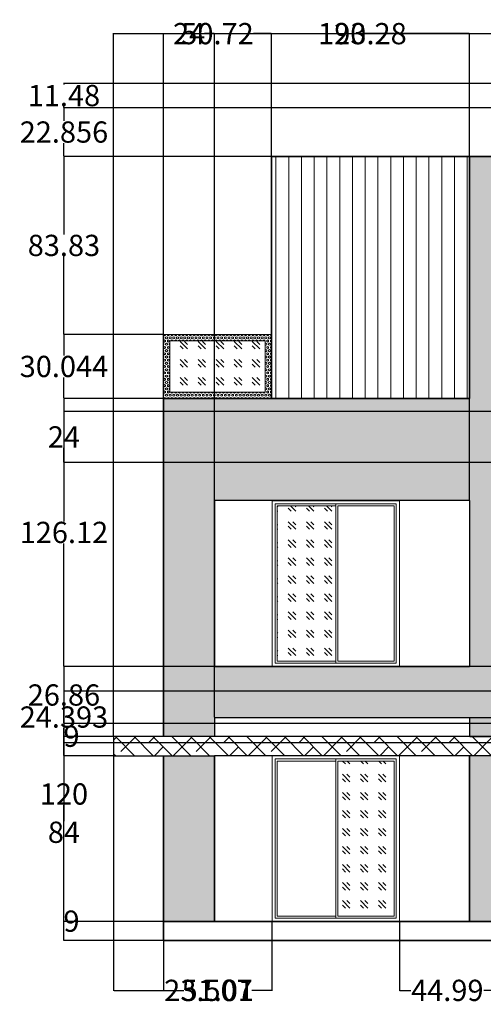
# Model space of a CAD drawing. Units: inches. Extents: x -37 to 519, y -28 to 435.
# Tile 1 of 3: x -37 to 182, y -28 to 435. Entities that reach past the tile are written whole.
import ezdxf

# ---------------------------------------------------------------- set-up
doc = ezdxf.new("R2010")
doc.units = ezdxf.units.IN
doc.header["$MEASUREMENT"] = 0
for name, color, linetype, lineweight in [('A-ANNO-DIMS', 2, 'Continuous', 18), ('A-GLAZ', 4, 'Continuous', 18), ('A-GLAZ-PATT', 9, 'Continuous', 13), ('A-WALL', 7, 'Continuous', 35), ('A-WALL-PATT', 8, 'Continuous', 13), ('A-WALL-TRIM', 7, 'Continuous', 25), ('A-WALL-TRIM-PATT', 8, 'Continuous', 13)]:
    doc.layers.add(name, color=color, linetype=linetype, lineweight=lineweight)
doc.styles.get("Standard").update_dxf_attribs({"font": 'arial.ttf'})
doc.dimstyles.get("Standard").update_dxf_attribs({"dimtxt": 10, "dimasz": 0.18, "dimexe": 0.18, "dimexo": 0.0625, "dimgap": 0.09, "dimtad": 0, "dimtih": 1, "dimtoh": 1, "dimdec": 0, "dimzin": 0, "dimdsep": 46, "dimlunit": 3, "dimtxsty": 'Standard', "dimcen": 0.09, "dimadec": 0, "dimazin": 0, "dimtfac": 1, "dimtdec": 0, "dimtofl": 0, "dimtmove": 0, "dimatfit": 3, "dimfxl": 1, "dimtolj": 1, "dimtzin": 0, "dimarcsym": 0})

# ---------------------------------------------------------------- blocks, each defined once
blk = doc.blocks.new('WIN-ALUM-60X78-ELEV')
for p, q in [((1.5, 1.5), (1.5, 76.5)), ((1.5, 76.5), (30, 76.5)), ((30, 1.5), (30, 76.5)), ((30, 76.5), (58.5, 76.5)), ((58.5, 76.5), (58.5, 1.5)), ((30, 1.5), (1.5, 1.5)), ((58.5, 1.5), (30, 1.5))]:
    blk.add_line(p, q)
blk.add_lwpolyline([(0, 0), (0, 78), (60, 78), (60, 0)], close=True)
for points in [[(29, 75.5), (29, 2.5), (2.5, 2.5), (2.5, 75.5), (29, 75.5)], [(30, 75.5), (57.5, 75.5), (57.5, 2.5), (30, 2.5)]]:
    blk.add_lwpolyline(points)
blk = doc.blocks.new('*D7')
at = {"layer": 'A-ANNO-DIMS', "color": 0, "lineweight": -2, "transparency": 16777216}
for p, q in [((7.62, 97.72), (7.62, 428.56)), ((7.8, 428.38), (224.17, 428.38)), ((474.95, 428.38), (258.57, 428.38)), ((475.13, 97.72), (475.13, 428.56))]:
    blk.add_line(p, q, dxfattribs=at)
at = {"layer": 'A-ANNO-DIMS', "color": 0, "transparency": 16777216}
for points in [[(7.8, 428.41), (7.8, 428.35), (7.62, 428.38)], [(474.95, 428.41), (474.95, 428.35), (475.13, 428.38)]]:
    blk.add_solid(points, dxfattribs=at)
at = {"layer": 'Defpoints', "color": 0, "transparency": 16777216}
for p in [(475.13, 428.38), (7.62, 97.65), (475.13, 97.65)]:
    blk.add_point(p, dxfattribs=at)
at = {"layer": 'A-ANNO-DIMS', "color": 0, "transparency": 16777216, "insert": (241.37, 428.38), "char_height": 10, "attachment_point": 5}
blk.add_mtext('\\A1;467.5', dxfattribs=at)
blk = doc.blocks.new('*D9')
at = {"layer": 'A-ANNO-DIMS', "color": 0, "lineweight": -2, "transparency": 16777216}
for p, q in [((7.62, 88.59), (7.62, -21.92)), ((31.13, 1.59), (31.13, -21.92)), ((7.8, -21.74), (30.95, -21.74)), ((31.13, -21.74), (31.31, -21.74))]:
    blk.add_line(p, q, dxfattribs=at)
at = {"layer": 'A-ANNO-DIMS', "color": 0, "transparency": 16777216}
for points in [[(7.8, -21.71), (7.8, -21.77), (7.62, -21.74)], [(30.95, -21.71), (30.95, -21.77), (31.13, -21.74)]]:
    blk.add_solid(points, dxfattribs=at)
at = {"layer": 'Defpoints', "color": 0, "transparency": 16777216}
for p in [(7.62, 88.65), (31.13, 1.65), (31.13, -21.74)]:
    blk.add_point(p, dxfattribs=at)
at = {"layer": 'A-ANNO-DIMS', "color": 0, "transparency": 16777216, "insert": (52.24, -21.74), "char_height": 10, "attachment_point": 5}
blk.add_mtext('\\A1;23.507', dxfattribs=at)
blk = doc.blocks.new('*D10')
at = {"layer": 'A-ANNO-DIMS', "color": 0, "lineweight": -2, "transparency": 16777216}
for p, q in [((31.13, 10.59), (31.13, -21.92)), ((82.13, 10.59), (82.13, -21.92)), ((31.31, -21.74), (40.63, -21.74)), ((81.95, -21.74), (72.63, -21.74))]:
    blk.add_line(p, q, dxfattribs=at)
at = {"layer": 'A-ANNO-DIMS', "color": 0, "transparency": 16777216}
for points in [[(31.31, -21.71), (31.31, -21.77), (31.13, -21.74)], [(81.95, -21.71), (81.95, -21.77), (82.13, -21.74)]]:
    blk.add_solid(points, dxfattribs=at)
at = {"layer": 'Defpoints', "color": 0, "transparency": 16777216}
for p in [(31.13, 10.65), (82.13, 10.65), (82.13, -21.74)]:
    blk.add_point(p, dxfattribs=at)
at = {"layer": 'A-ANNO-DIMS', "color": 0, "transparency": 16777216, "insert": (56.63, -21.74), "char_height": 10, "attachment_point": 5}
blk.add_mtext('\\A1;51.01', dxfattribs=at)
blk = doc.blocks.new('*D11')
at = {"layer": 'A-ANNO-DIMS', "color": 0, "lineweight": -2, "transparency": 16777216}
for p, q in [((142.13, 10.59), (142.13, -21.92)), ((187.13, 10.59), (187.13, -21.92)), ((142.31, -21.74), (147.46, -21.74)), ((186.95, -21.74), (181.8, -21.74))]:
    blk.add_line(p, q, dxfattribs=at)
at = {"layer": 'A-ANNO-DIMS', "color": 0, "transparency": 16777216}
for points in [[(142.31, -21.71), (142.31, -21.77), (142.13, -21.74)], [(186.95, -21.71), (186.95, -21.77), (187.13, -21.74)]]:
    blk.add_solid(points, dxfattribs=at)
at = {"layer": 'Defpoints', "color": 0, "transparency": 16777216}
for p in [(142.13, 10.65), (187.13, 10.65), (187.13, -21.74)]:
    blk.add_point(p, dxfattribs=at)
at = {"layer": 'A-ANNO-DIMS', "color": 0, "transparency": 16777216, "insert": (164.63, -21.74), "char_height": 10, "attachment_point": 5}
blk.add_mtext('\\A1;44.99', dxfattribs=at)
blk = doc.blocks.new('*D16')
at = {"layer": 'A-ANNO-DIMS', "color": 0, "lineweight": -2, "transparency": 16777216}
for p, q in [((206.27, 94.65), (-15.95, 94.65)), ((-15.77, 94.47), (-15.77, 57.85)), ((-15.77, 10.83), (-15.77, 47.46)), ((206.27, 10.65), (-15.95, 10.65))]:
    blk.add_line(p, q, dxfattribs=at)
at = {"layer": 'A-ANNO-DIMS', "color": 0, "transparency": 16777216}
for points in [[(-15.8, 94.47), (-15.74, 94.47), (-15.77, 94.65)], [(-15.8, 10.83), (-15.74, 10.83), (-15.77, 10.65)]]:
    blk.add_solid(points, dxfattribs=at)
at = {"layer": 'Defpoints', "color": 0, "transparency": 16777216}
for p in [(-15.77, 94.65), (206.33, 94.65), (206.33, 10.65)]:
    blk.add_point(p, dxfattribs=at)
at = {"layer": 'A-ANNO-DIMS', "color": 0, "transparency": 16777216, "insert": (-15.77, 52.65), "char_height": 10, "attachment_point": 5}
blk.add_mtext('\\A1;84', dxfattribs=at)
blk = doc.blocks.new('*D18')
at = {"layer": 'A-ANNO-DIMS', "color": 0, "lineweight": -2, "transparency": 16777216}
for p, q in [((31.06, 10.65), (-15.95, 10.65)), ((-15.77, 10.65), (-15.77, 10.83)), ((-15.77, 10.83), (-15.59, 10.83)), ((-15.77, 1.83), (-15.77, 10.47)), ((31.06, 1.65), (-15.95, 1.65))]:
    blk.add_line(p, q, dxfattribs=at)
at = {"layer": 'A-ANNO-DIMS', "color": 0, "transparency": 16777216}
for points in [[(-15.8, 10.47), (-15.74, 10.47), (-15.77, 10.65)], [(-15.8, 1.83), (-15.74, 1.83), (-15.77, 1.65)]]:
    blk.add_solid(points, dxfattribs=at)
at = {"layer": 'Defpoints', "color": 0, "transparency": 16777216}
for p in [(-15.77, 10.65), (31.13, 10.65), (31.13, 1.65)]:
    blk.add_point(p, dxfattribs=at)
at = {"layer": 'A-ANNO-DIMS', "color": 0, "transparency": 16777216, "insert": (-12.21, 10.83), "char_height": 10, "attachment_point": 5}
blk.add_mtext('\\A1;9', dxfattribs=at)
blk = doc.blocks.new('*D19')
at = {"layer": 'A-ANNO-DIMS', "color": 0, "lineweight": -2, "transparency": 16777216}
for p, q in [((82.07, 130.65), (-15.95, 130.65)), ((-15.77, 130.47), (-15.77, 75.85)), ((-15.77, 10.83), (-15.77, 65.46)), ((31.06, 10.65), (-15.95, 10.65))]:
    blk.add_line(p, q, dxfattribs=at)
at = {"layer": 'A-ANNO-DIMS', "color": 0, "transparency": 16777216}
for points in [[(-15.8, 130.47), (-15.74, 130.47), (-15.77, 130.65)], [(-15.8, 10.83), (-15.74, 10.83), (-15.77, 10.65)]]:
    blk.add_solid(points, dxfattribs=at)
at = {"layer": 'Defpoints', "color": 0, "transparency": 16777216}
for p in [(-15.77, 130.65), (82.13, 130.65), (31.13, 10.65)]:
    blk.add_point(p, dxfattribs=at)
at = {"layer": 'A-ANNO-DIMS', "color": 0, "transparency": 16777216, "insert": (-15.77, 70.65), "char_height": 10, "attachment_point": 5}
blk.add_mtext('\\A1;120', dxfattribs=at)
blk = doc.blocks.new('*D20')
at = {"layer": 'A-ANNO-DIMS', "color": 0, "lineweight": -2, "transparency": 16777216}
for p, q in [((31.06, 256.78), (-15.95, 256.78)), ((-15.77, 256.6), (-15.77, 198.91)), ((-15.77, 130.83), (-15.77, 188.52)), ((82.07, 130.65), (-15.95, 130.65))]:
    blk.add_line(p, q, dxfattribs=at)
at = {"layer": 'A-ANNO-DIMS', "color": 0, "transparency": 16777216}
for points in [[(-15.8, 256.6), (-15.74, 256.6), (-15.77, 256.78)], [(-15.8, 130.83), (-15.74, 130.83), (-15.77, 130.65)]]:
    blk.add_solid(points, dxfattribs=at)
at = {"layer": 'Defpoints', "color": 0, "transparency": 16777216}
for p in [(-15.77, 256.78), (31.13, 256.78), (82.13, 130.65)]:
    blk.add_point(p, dxfattribs=at)
at = {"layer": 'A-ANNO-DIMS', "color": 0, "transparency": 16777216, "insert": (-15.77, 193.71), "char_height": 10, "attachment_point": 5}
blk.add_mtext('\\A1;126.12', dxfattribs=at)
blk = doc.blocks.new('*D21')
at = {"layer": 'A-ANNO-DIMS', "color": 0, "lineweight": -2, "transparency": 16777216}
for p, q in [((31.06, 286.82), (-15.95, 286.82)), ((-15.77, 286.64), (-15.77, 277)), ((-15.77, 256.96), (-15.77, 266.6)), ((31.06, 256.78), (-15.95, 256.78))]:
    blk.add_line(p, q, dxfattribs=at)
at = {"layer": 'A-ANNO-DIMS', "color": 0, "transparency": 16777216}
for points in [[(-15.8, 286.64), (-15.74, 286.64), (-15.77, 286.82)], [(-15.8, 256.96), (-15.74, 256.96), (-15.77, 256.78)]]:
    blk.add_solid(points, dxfattribs=at)
at = {"layer": 'Defpoints', "color": 0, "transparency": 16777216}
for p in [(-15.77, 286.82), (31.13, 286.82), (31.13, 256.78)]:
    blk.add_point(p, dxfattribs=at)
at = {"layer": 'A-ANNO-DIMS', "color": 0, "transparency": 16777216, "insert": (-15.77, 271.8), "char_height": 10, "attachment_point": 5}
blk.add_mtext('\\A1;30.044', dxfattribs=at)
blk = doc.blocks.new('*D22')
at = {"layer": 'A-ANNO-DIMS', "color": 0, "lineweight": -2, "transparency": 16777216}
for p, q in [((81.79, 370.65), (-15.95, 370.65)), ((-15.77, 370.47), (-15.77, 333.94)), ((-15.77, 287), (-15.77, 323.54)), ((31.06, 286.82), (-15.95, 286.82))]:
    blk.add_line(p, q, dxfattribs=at)
at = {"layer": 'A-ANNO-DIMS', "color": 0, "transparency": 16777216}
for points in [[(-15.8, 370.47), (-15.74, 370.47), (-15.77, 370.65)], [(-15.8, 287), (-15.74, 287), (-15.77, 286.82)]]:
    blk.add_solid(points, dxfattribs=at)
at = {"layer": 'Defpoints', "color": 0, "transparency": 16777216}
for p in [(-15.77, 370.65), (81.85, 370.65), (31.13, 286.82)]:
    blk.add_point(p, dxfattribs=at)
at = {"layer": 'A-ANNO-DIMS', "color": 0, "transparency": 16777216, "insert": (-15.77, 328.74), "char_height": 10, "attachment_point": 5}
blk.add_mtext('\\A1;83.83', dxfattribs=at)
blk = doc.blocks.new('*D23')
at = {"layer": 'A-ANNO-DIMS', "color": 0, "lineweight": -2, "transparency": 16777216}
for p, q in [((31.13, 286.88), (31.13, 428.56)), ((31.31, 428.38), (39.58, 428.38)), ((81.67, 428.38), (73.4, 428.38)), ((81.85, 370.72), (81.85, 428.56))]:
    blk.add_line(p, q, dxfattribs=at)
at = {"layer": 'A-ANNO-DIMS', "color": 0, "transparency": 16777216}
for points in [[(31.31, 428.41), (31.31, 428.35), (31.13, 428.38)], [(81.67, 428.41), (81.67, 428.35), (81.85, 428.38)]]:
    blk.add_solid(points, dxfattribs=at)
at = {"layer": 'Defpoints', "color": 0, "transparency": 16777216}
for p in [(81.85, 428.38), (81.85, 370.65), (31.13, 286.82)]:
    blk.add_point(p, dxfattribs=at)
at = {"layer": 'A-ANNO-DIMS', "color": 0, "transparency": 16777216, "insert": (56.49, 428.38), "char_height": 10, "attachment_point": 5}
blk.add_mtext('\\A1;50.72', dxfattribs=at)
blk = doc.blocks.new('*D24')
at = {"layer": 'A-ANNO-DIMS', "color": 0, "lineweight": -2, "transparency": 16777216}
for p, q in [((81.85, 370.72), (81.85, 428.56)), ((82.03, 428.38), (111.52, 428.38)), ((174.95, 428.38), (145.46, 428.38)), ((175.13, 370.72), (175.13, 428.56))]:
    blk.add_line(p, q, dxfattribs=at)
at = {"layer": 'A-ANNO-DIMS', "color": 0, "transparency": 16777216}
for points in [[(82.03, 428.41), (82.03, 428.35), (81.85, 428.38)], [(174.95, 428.41), (174.95, 428.35), (175.13, 428.38)]]:
    blk.add_solid(points, dxfattribs=at)
at = {"layer": 'Defpoints', "color": 0, "transparency": 16777216}
for p in [(175.13, 428.38), (81.85, 370.65), (175.13, 370.65)]:
    blk.add_point(p, dxfattribs=at)
at = {"layer": 'A-ANNO-DIMS', "color": 0, "transparency": 16777216, "insert": (128.49, 428.38), "char_height": 10, "attachment_point": 5}
blk.add_mtext('\\A1;93.28', dxfattribs=at)
blk = doc.blocks.new('*D27')
at = {"layer": 'A-ANNO-DIMS', "color": 0, "lineweight": -2, "transparency": 16777216}
for p, q in [((295.06, 119.05), (-15.95, 119.05)), ((-15.77, 118.87), (-15.77, 112.05)), ((-15.77, 94.83), (-15.77, 101.65)), ((266, 94.65), (-15.95, 94.65))]:
    blk.add_line(p, q, dxfattribs=at)
at = {"layer": 'A-ANNO-DIMS', "color": 0, "transparency": 16777216}
for points in [[(-15.8, 118.87), (-15.74, 118.87), (-15.77, 119.05)], [(-15.8, 94.83), (-15.74, 94.83), (-15.77, 94.65)]]:
    blk.add_solid(points, dxfattribs=at)
at = {"layer": 'Defpoints', "color": 0, "transparency": 16777216}
for p in [(-15.77, 119.05), (295.13, 119.05), (266.06, 94.65)]:
    blk.add_point(p, dxfattribs=at)
at = {"layer": 'A-ANNO-DIMS', "color": 0, "transparency": 16777216, "insert": (-15.77, 106.85), "char_height": 10, "attachment_point": 5}
blk.add_mtext('\\A1;24.393', dxfattribs=at)
blk = doc.blocks.new('*D28')
at = {"layer": 'A-ANNO-DIMS', "color": 0, "lineweight": -2, "transparency": 16777216}
for p, q in [((7.56, 97.65), (-15.95, 97.65)), ((-15.77, 97.65), (-15.77, 97.83)), ((-15.77, 97.83), (-15.59, 97.83)), ((-15.77, 88.83), (-15.77, 97.47)), ((7.56, 88.65), (-15.95, 88.65))]:
    blk.add_line(p, q, dxfattribs=at)
at = {"layer": 'A-ANNO-DIMS', "color": 0, "transparency": 16777216}
for points in [[(-15.8, 97.47), (-15.74, 97.47), (-15.77, 97.65)], [(-15.8, 88.83), (-15.74, 88.83), (-15.77, 88.65)]]:
    blk.add_solid(points, dxfattribs=at)
at = {"layer": 'Defpoints', "color": 0, "transparency": 16777216}
for p in [(-15.77, 97.65), (7.62, 97.65), (7.62, 88.65)]:
    blk.add_point(p, dxfattribs=at)
at = {"layer": 'A-ANNO-DIMS', "color": 0, "transparency": 16777216, "insert": (-12.21, 97.83), "char_height": 10, "attachment_point": 5}
blk.add_mtext('\\A1;9', dxfattribs=at)
blk = doc.blocks.new('*D29')
at = {"layer": 'A-ANNO-DIMS', "color": 0, "lineweight": -2, "transparency": 16777216}
for p, q in [((55.13, 208.84), (55.13, 428.56)), ((55.31, 428.38), (104.48, 428.38)), ((174.95, 428.38), (125.78, 428.38)), ((175.13, 208.84), (175.13, 428.56))]:
    blk.add_line(p, q, dxfattribs=at)
at = {"layer": 'A-ANNO-DIMS', "color": 0, "transparency": 16777216}
for points in [[(55.31, 428.41), (55.31, 428.35), (55.13, 428.38)], [(174.95, 428.41), (174.95, 428.35), (175.13, 428.38)]]:
    blk.add_solid(points, dxfattribs=at)
at = {"layer": 'Defpoints', "color": 0, "transparency": 16777216}
for p in [(175.13, 428.38), (55.13, 208.78), (175.13, 208.78)]:
    blk.add_point(p, dxfattribs=at)
at = {"layer": 'A-ANNO-DIMS', "color": 0, "transparency": 16777216, "insert": (115.13, 428.38), "char_height": 10, "attachment_point": 5}
blk.add_mtext('\\A1;120', dxfattribs=at)
blk = doc.blocks.new('*D30')
at = {"layer": 'A-ANNO-DIMS', "color": 0, "lineweight": -2, "transparency": 16777216}
for p, q in [((31.13, 97.72), (31.13, 428.56)), ((31.31, 428.38), (35.81, 428.38)), ((54.95, 428.38), (50.44, 428.38)), ((55.13, 106.72), (55.13, 428.56))]:
    blk.add_line(p, q, dxfattribs=at)
at = {"layer": 'A-ANNO-DIMS', "color": 0, "transparency": 16777216}
for points in [[(31.31, 428.41), (31.31, 428.35), (31.13, 428.38)], [(54.95, 428.41), (54.95, 428.35), (55.13, 428.38)]]:
    blk.add_solid(points, dxfattribs=at)
at = {"layer": 'Defpoints', "color": 0, "transparency": 16777216}
for p in [(55.13, 428.38), (55.13, 106.65), (31.13, 97.65)]:
    blk.add_point(p, dxfattribs=at)
at = {"layer": 'A-ANNO-DIMS', "color": 0, "transparency": 16777216, "insert": (43.13, 428.38), "char_height": 10, "attachment_point": 5}
blk.add_mtext('\\A1;24', dxfattribs=at)
blk = doc.blocks.new('*D31')
at = {"layer": 'A-ANNO-DIMS', "color": 0, "lineweight": -2, "transparency": 16777216}
for p, q in [((175.19, 106.65), (498.7, 106.65)), ((498.52, 106.65), (498.52, 106.83)), ((498.52, 106.83), (498.7, 106.83)), ((498.52, 97.83), (498.52, 106.47)), ((175.19, 97.65), (498.7, 97.65))]:
    blk.add_line(p, q, dxfattribs=at)
at = {"layer": 'A-ANNO-DIMS', "color": 0, "transparency": 16777216}
for points in [[(498.49, 106.47), (498.55, 106.47), (498.52, 106.65)], [(498.49, 97.83), (498.55, 97.83), (498.52, 97.65)]]:
    blk.add_solid(points, dxfattribs=at)
at = {"layer": 'Defpoints', "color": 0, "transparency": 16777216}
for p in [(175.13, 106.65), (498.52, 106.65), (175.13, 97.65)]:
    blk.add_point(p, dxfattribs=at)
at = {"layer": 'A-ANNO-DIMS', "color": 0, "transparency": 16777216, "insert": (502.08, 106.83), "char_height": 10, "attachment_point": 5}
blk.add_mtext('\\A1;9', dxfattribs=at)
blk = doc.blocks.new('*D33')
at = {"layer": 'A-ANNO-DIMS', "color": 0, "lineweight": -2, "transparency": 16777216}
for p, q in [((319.06, 250.65), (-15.95, 250.65)), ((-15.77, 250.47), (-15.77, 243.76)), ((-15.77, 226.83), (-15.77, 233.54)), ((295.06, 226.65), (-15.95, 226.65))]:
    blk.add_line(p, q, dxfattribs=at)
at = {"layer": 'A-ANNO-DIMS', "color": 0, "transparency": 16777216}
for points in [[(-15.8, 250.47), (-15.74, 250.47), (-15.77, 250.65)], [(-15.8, 226.83), (-15.74, 226.83), (-15.77, 226.65)]]:
    blk.add_solid(points, dxfattribs=at)
at = {"layer": 'Defpoints', "color": 0, "transparency": 16777216}
for p in [(319.13, 250.65), (-15.77, 226.65), (295.13, 226.65)]:
    blk.add_point(p, dxfattribs=at)
at = {"layer": 'A-ANNO-DIMS', "color": 0, "transparency": 16777216, "insert": (-15.77, 238.65), "char_height": 10, "attachment_point": 5}
blk.add_mtext('\\A1;24', dxfattribs=at)
blk = doc.blocks.new('*D42')
at = {"layer": 'A-ANNO-DIMS', "color": 0, "lineweight": -2, "transparency": 16777216}
for p, q in [((312.44, 393.51), (-15.95, 393.51)), ((-15.77, 393.33), (-15.77, 387.28)), ((-15.77, 370.83), (-15.77, 376.89)), ((312.44, 370.65), (-15.95, 370.65))]:
    blk.add_line(p, q, dxfattribs=at)
at = {"layer": 'A-ANNO-DIMS', "color": 0, "transparency": 16777216}
for points in [[(-15.8, 393.33), (-15.74, 393.33), (-15.77, 393.51)], [(-15.8, 370.83), (-15.74, 370.83), (-15.77, 370.65)]]:
    blk.add_solid(points, dxfattribs=at)
at = {"layer": 'Defpoints', "color": 0, "transparency": 16777216}
for p in [(-15.77, 393.51), (312.5, 393.51), (312.5, 370.65)]:
    blk.add_point(p, dxfattribs=at)
at = {"layer": 'A-ANNO-DIMS', "color": 0, "transparency": 16777216, "insert": (-15.77, 382.08), "char_height": 10, "attachment_point": 5}
blk.add_mtext('\\A1;22.856', dxfattribs=at)
blk = doc.blocks.new('*D43')
at = {"layer": 'A-ANNO-DIMS', "color": 0, "lineweight": -2, "transparency": 16777216}
for p, q in [((295.06, 404.99), (-15.95, 404.99)), ((-15.77, 404.81), (-15.77, 404.44)), ((-15.77, 393.69), (-15.77, 394.05)), ((295.06, 393.51), (-15.95, 393.51))]:
    blk.add_line(p, q, dxfattribs=at)
at = {"layer": 'A-ANNO-DIMS', "color": 0, "transparency": 16777216}
for points in [[(-15.8, 404.81), (-15.74, 404.81), (-15.77, 404.99)], [(-15.8, 393.69), (-15.74, 393.69), (-15.77, 393.51)]]:
    blk.add_solid(points, dxfattribs=at)
at = {"layer": 'Defpoints', "color": 0, "transparency": 16777216}
for p in [(-15.77, 404.99), (295.13, 404.99), (295.13, 393.51)]:
    blk.add_point(p, dxfattribs=at)
at = {"layer": 'A-ANNO-DIMS', "color": 0, "transparency": 16777216, "insert": (-15.77, 399.25), "char_height": 10, "attachment_point": 5}
blk.add_mtext('\\A1;11.48', dxfattribs=at)
blk = doc.blocks.new('*D46')
at = {"layer": 'A-ANNO-DIMS', "color": 0, "lineweight": -2, "transparency": 16777216}
for p, q in [((307.06, 130.65), (-15.95, 130.65)), ((-15.77, 130.47), (-15.77, 122.42)), ((-15.77, 103.97), (-15.77, 112.03)), ((307.06, 103.79), (-15.95, 103.79))]:
    blk.add_line(p, q, dxfattribs=at)
at = {"layer": 'A-ANNO-DIMS', "color": 0, "transparency": 16777216}
for points in [[(-15.8, 130.47), (-15.74, 130.47), (-15.77, 130.65)], [(-15.8, 103.97), (-15.74, 103.97), (-15.77, 103.79)]]:
    blk.add_solid(points, dxfattribs=at)
at = {"layer": 'Defpoints', "color": 0, "transparency": 16777216}
for p in [(307.13, 130.65), (-15.77, 103.79), (307.13, 103.79)]:
    blk.add_point(p, dxfattribs=at)
at = {"layer": 'A-ANNO-DIMS', "color": 0, "transparency": 16777216, "insert": (-15.77, 117.22), "char_height": 10, "attachment_point": 5}
blk.add_mtext('\\A1;26.86', dxfattribs=at)

msp = doc.modelspace()

# ---------------------------------------------------------------- hatches: boundary and pattern name
at = {"layer": 'A-GLAZ-PATT'}
h = msp.add_hatch(dxfattribs=at)
h.set_pattern_fill('GOST_GLASS', color=256, angle=90)
h.set_pattern_definition([(135, (0, 0), (5e-16, 8.48528), [5, -7]), (135, (1e-16, 2.1213), (5e-16, 8.48528), [2, -10]), (135, (-2.1213, 1e-16), (5e-16, 8.48528), [2, -10])])
h.paths.add_polyline_path([(112.1341, 206.153), (84.6341, 206.153), (84.6341, 133.153), (112.1341, 133.153)])
h.paths.add_polyline_path([(139.6341, 86.153), (113.1341, 86.153), (113.1341, 13.153), (139.6341, 13.153)])
h.paths.add_polyline_path([(369.1204, 86.153), (342.6204, 86.153), (342.6204, 13.153), (369.1204, 13.153)])
h.paths.add_polyline_path([(391.6341, 206.153), (365.1341, 206.153), (365.1341, 133.153), (391.6341, 133.153)])
h.paths.add_polyline_path([(78.851, 283.8209), (34.1272, 283.8209), (34.1272, 259.7765), (78.851, 259.7765)])
at = {"layer": 'A-WALL-PATT'}
h = msp.add_hatch(color=256, dxfattribs=at)
h.dxf.hatch_style = 1
h.paths.add_polyline_path([(451.1272, 370.653), (295.1272, 370.653), (295.1272, 226.653), (451.1272, 226.653)])
h.paths.add_polyline_path([(319.1272, 346.653), (427.1272, 346.653), (427.1272, 250.653), (319.1272, 250.653)], flags=16)
h.paths.add_polyline_path([(334.1341, 346.653), (394.1341, 346.653), (394.1341, 250.653), (334.1341, 250.653)], flags=0)
h.paths.add_polyline_path([(335.6341, 345.153), (364.1341, 345.153), (392.6341, 345.153), (392.6341, 252.153), (364.1341, 252.153), (335.6341, 252.153)], flags=0)
h.paths.add_polyline_path([(336.6341, 344.153), (364.1341, 344.153), (364.1341, 253.153), (336.6341, 253.153)], flags=0)
h.paths.add_polyline_path([(365.1341, 344.153), (391.6341, 344.153), (391.6341, 253.153), (365.1341, 253.153)], flags=0)
h.paths.add_polyline_path([(187.1272, 370.653), (175.1272, 370.653), (175.1272, 256.7765), (31.1272, 256.7765), (31.1272, 97.653), (55.1272, 97.653), (55.1272, 106.653), (175.1272, 106.653), (175.1272, 97.653), (187.1272, 97.653)])
h.paths.add_polyline_path([(175.1272, 208.7765), (175.1272, 130.653), (55.1272, 130.653), (55.1272, 208.7765)], flags=16)
h.paths.add_polyline_path([(142.1341, 208.653), (142.1341, 130.653), (82.1341, 130.653), (82.1341, 208.653)], flags=0)
h.paths.add_polyline_path([(112.1341, 207.153), (140.6341, 207.153), (140.6341, 132.153), (112.1341, 132.153), (83.6341, 132.153), (83.6341, 207.153)], flags=0)
h.paths.add_polyline_path([(112.1341, 133.153), (84.6341, 133.153), (84.6341, 206.153), (112.1341, 206.153)], flags=0)
h.paths.add_polyline_path([(139.6341, 206.153), (139.6341, 133.153), (113.1341, 133.153), (113.1341, 206.153)], flags=0)
h.paths.add_polyline_path([(187.1272, 88.653), (175.1272, 88.653), (175.1272, 10.653), (187.1272, 10.653)])
h.paths.add_polyline_path([(307.1272, 88.653), (295.1272, 88.653), (295.1272, 10.653), (307.1272, 10.653)])
h.paths.add_polyline_path([(451.1272, 88.653), (427.1272, 88.653), (427.1272, 10.653), (451.1272, 10.653)])
h = msp.add_hatch(dxfattribs=at)
h.set_pattern_fill('_USER', color=256, scale=6, angle=90, pattern_type=0)
h.set_pattern_definition([(90, (0, 0), (-6, 4e-16), [])])
h.paths.add_polyline_path([(175.1272, 370.653), (81.851, 370.653), (81.851, 256.7765), (175.1272, 256.7765)])
h = msp.add_hatch(color=256, dxfattribs=at)
h.dxf.hatch_style = 1
h.paths.add_polyline_path([(307.1272, 226.653), (295.1272, 226.653), (295.1272, 97.653), (307.1272, 97.653), (307.1272, 130.653)])
h.paths.add_polyline_path([(55.1272, 88.653), (31.1272, 88.653), (31.1272, 10.653), (55.1272, 10.653)])
at = {"layer": 'A-WALL-TRIM-PATT'}
h = msp.add_hatch(dxfattribs=at)
h.set_pattern_fill('HEX', color=256, scale=4, angle=90)
h.paths.add_polyline_path([(81.851, 286.8209), (31.1272, 286.8209), (31.1272, 256.7765), (81.851, 256.7765)])
h.paths.add_polyline_path([(78.851, 283.8209), (78.851, 259.7765), (34.1272, 259.7765), (34.1272, 283.8209)], flags=16)
h = msp.add_hatch(dxfattribs=at)
h.set_pattern_fill('ANSI38', color=256, scale=50, angle=90)
h.paths.add_polyline_path([(187.1272, 97.653), (55.1272, 97.653), (7.6202, 97.653), (7.6202, 88.653), (55.1272, 88.653), (187.1272, 88.653)])
h.paths.add_polyline_path([(475.1272, 97.653), (427.1272, 97.653), (295.1272, 97.653), (295.1272, 88.653), (427.1272, 88.653), (475.1272, 88.653)])

# ---------------------------------------------------------------- linework, layer by layer
at = {"layer": 'A-GLAZ'}
for p, q in [((112.1341, 207.153), (83.6341, 207.153)), ((83.6341, 207.153), (83.6341, 132.153)), ((112.1341, 132.153), (112.1341, 207.153)), ((140.6341, 207.153), (112.1341, 207.153)), ((140.6341, 132.153), (140.6341, 207.153)), ((83.6341, 132.153), (112.1341, 132.153)), ((112.1341, 132.153), (140.6341, 132.153)), ((112.1341, 87.153), (83.6341, 87.153)), ((83.6341, 87.153), (83.6341, 12.153)), ((112.1341, 12.153), (112.1341, 87.153)), ((140.6341, 87.153), (112.1341, 87.153)), ((140.6341, 12.153), (140.6341, 87.153)), ((83.6341, 12.153), (112.1341, 12.153)), ((112.1341, 12.153), (140.6341, 12.153))]:
    msp.add_line(p, q, dxfattribs=at)
for points in [[(81.851, 286.8209), (31.1272, 286.8209), (31.1272, 256.7765), (81.851, 256.7765)], [(78.851, 283.8209), (34.1272, 283.8209), (34.1272, 259.7765), (78.851, 259.7765)], [(142.1341, 130.653), (142.1341, 208.653), (82.1341, 208.653), (82.1341, 130.653)], [(142.1341, 10.653), (142.1341, 88.653), (82.1341, 88.653), (82.1341, 10.653)]]:
    msp.add_lwpolyline(points, close=True, dxfattribs=at)
for points in [[(112.1341, 206.153), (84.6341, 206.153), (84.6341, 133.153), (112.1341, 133.153)], [(113.1341, 206.153), (113.1341, 133.153), (139.6341, 133.153), (139.6341, 206.153), (113.1341, 206.153)], [(112.1341, 86.153), (84.6341, 86.153), (84.6341, 13.153), (112.1341, 13.153)], [(113.1341, 86.153), (113.1341, 13.153), (139.6341, 13.153), (139.6341, 86.153), (113.1341, 86.153)]]:
    msp.add_lwpolyline(points, dxfattribs=at)
at = {"layer": 'A-WALL'}
for p, q in [((81.851, 370.653), (81.851, 256.7765)), ((187.1272, 370.653), (81.851, 370.653)), ((175.1272, 370.653), (175.1272, 256.7765)), ((31.1272, 256.7765), (31.1272, 97.653)), ((175.1272, 256.7765), (31.1272, 256.7765)), ((31.1272, 88.653), (31.1272, 1.653)), ((55.1272, 88.653), (55.1272, 10.653)), ((175.1272, 88.653), (175.1272, 10.653)), ((31.1272, 10.653), (451.1272, 10.653)), ((31.1272, 1.653), (451.1272, 1.653))]:
    msp.add_line(p, q, dxfattribs=at)
at = {"layer": 'A-WALL-TRIM'}
for p, q in [((55.1272, 208.7765), (55.1272, 130.653)), ((175.1272, 208.7765), (55.1272, 208.7765)), ((175.1272, 208.7765), (175.1272, 130.653)), ((55.1272, 130.653), (163.1272, 130.653)), ((55.1272, 130.653), (175.1272, 130.653)), ((55.1272, 106.653), (163.1272, 106.653)), ((55.1272, 106.653), (175.1272, 106.653)), ((55.1272, 106.653), (55.1272, 97.653)), ((175.1272, 106.653), (175.1272, 97.653)), ((187.1272, 97.653), (55.1272, 97.653)), ((187.1272, 88.653), (55.1272, 88.653))]:
    msp.add_line(p, q, dxfattribs=at)
msp.add_lwpolyline([(55.1272, 97.653), (7.6202, 97.653), (7.6202, 88.653), (55.1272, 88.653)], dxfattribs=at)

# ---------------------------------------------------------------- block references
at = {"layer": 'A-GLAZ', "extrusion": (0, 0, -1), "zscale": -1}
for p in [(-142.1341, 130.653), (-142.1341, 10.653)]:
    msp.add_blockref('WIN-ALUM-60X78-ELEV', p, dxfattribs=at)

# ---------------------------------------------------------------- dimensions: what is measured, and where the dimension line sits
at = {"layer": 'A-ANNO-DIMS'}
for base, p1, p2, override, picture, middle in [((475.1272, 428.3793), (7.6202, 97.653), (475.1272, 97.653), {"dimdec": 1, "dimlfac": 1, "dimrnd": 0, "dimzin": 0, "dimdsep": 46, "dimlunit": 2}, '*D7', (241.3737, 428.3793)), ((81.851, 428.3793), (31.1272, 286.8209), (81.851, 370.653), {"dimdec": 2, "dimlfac": 1, "dimrnd": 0, "dimzin": 0, "dimdsep": 46, "dimlunit": 2}, '*D23', (56.4891, 428.3793)), ((55.1272, 428.3793), (31.1272, 97.653), (55.1272, 106.653), {"dimdec": 0, "dimlfac": 1, "dimrnd": 0, "dimzin": 0, "dimdsep": 46, "dimlunit": 2}, '*D30', (43.1272, 428.3793)), ((175.1272, 428.3793), (55.1272, 208.7765), (175.1272, 208.7765), {"dimdec": 0, "dimlfac": 1, "dimrnd": 0, "dimzin": 0, "dimdsep": 46, "dimlunit": 2}, '*D29', (115.1272, 428.3793)), ((175.1272, 428.3793), (81.851, 370.653), (175.1272, 370.653), {"dimdec": 2, "dimlfac": 1, "dimrnd": 0, "dimzin": 0, "dimdsep": 46, "dimlunit": 2}, '*D24', (128.4891, 428.3793)), ((31.1272, -21.737), (7.6202, 88.653), (31.1272, 1.653), {"dimdec": 3, "dimlfac": 1, "dimrnd": 0, "dimzin": 0, "dimdsep": 46, "dimlunit": 2}, '*D9', (52.2397, -21.737)), ((82.1341, -21.737), (31.1272, 10.653), (82.1341, 10.653), {"dimdec": 2, "dimlfac": 1, "dimrnd": 0, "dimzin": 0, "dimdsep": 46, "dimlunit": 2}, '*D10', (56.6307, -21.737)), ((187.1272, -21.737), (142.1341, 10.653), (187.1272, 10.653), {"dimdec": 2, "dimlfac": 1, "dimrnd": 0, "dimzin": 0, "dimdsep": 46, "dimlunit": 2}, '*D11', (164.6307, -21.737))]:
    dim = msp.add_linear_dim(base=base, p1=p1, p2=p2, dimstyle='Standard', override=override, dxfattribs=at)
    dim.commit()
    dim.dimension.update_dxf_attribs({"geometry": picture, "text_midpoint": middle})
for base, p1, p2, override, picture, middle in [((-15.7698, 404.9893), (295.1272, 393.509), (295.1272, 404.9893), {"dimdec": 2, "dimlfac": 1, "dimrnd": 0, "dimzin": 0, "dimdsep": 46, "dimlunit": 2}, '*D43', (-15.7698, 399.2491)), ((-15.7698, 393.509), (312.5031, 370.653), (312.5031, 393.509), {"dimdec": 3, "dimlfac": 1, "dimrnd": 0, "dimzin": 0, "dimdsep": 46, "dimlunit": 2}, '*D42', (-15.7698, 382.081)), ((-15.7698, 370.653), (31.1272, 286.8209), (81.851, 370.653), {"dimdec": 2, "dimlfac": 1, "dimrnd": 0, "dimzin": 0, "dimdsep": 46, "dimlunit": 2}, '*D22', (-15.7698, 328.7369)), ((-15.7698, 286.8209), (31.1272, 256.7765), (31.1272, 286.8209), {"dimdec": 3, "dimlfac": 1, "dimrnd": 0, "dimzin": 0, "dimdsep": 46, "dimlunit": 2}, '*D21', (-15.7698, 271.7987)), ((-15.7698, 256.7765), (82.1341, 130.653), (31.1272, 256.7765), {"dimdec": 2, "dimlfac": 1, "dimrnd": 0, "dimzin": 0, "dimdsep": 46, "dimlunit": 2}, '*D20', (-15.7698, 193.7147)), ((-15.7698, 226.653), (319.1272, 250.653), (295.1272, 226.653), {"dimdec": 0, "dimlfac": 1, "dimrnd": 0, "dimzin": 0, "dimdsep": 46, "dimlunit": 2}, '*D33', (-15.7698, 238.653)), ((-15.7698, 103.7936), (307.1272, 130.653), (307.1272, 103.7936), {"dimdec": 2, "dimlfac": 1, "dimrnd": 0, "dimzin": 0, "dimdsep": 46, "dimlunit": 2}, '*D46', (-15.7698, 117.2233)), ((-15.7698, 130.653), (31.1272, 10.653), (82.1341, 130.653), {"dimdec": 0, "dimlfac": 1, "dimrnd": 0, "dimzin": 0, "dimdsep": 46, "dimlunit": 2}, '*D19', (-15.7698, 70.653)), ((-15.7698, 119.0462), (266.063, 94.653), (295.1272, 119.0462), {"dimdec": 3, "dimlfac": 1, "dimrnd": 0, "dimzin": 0, "dimdsep": 46, "dimlunit": 2}, '*D27', (-15.7698, 106.8496)), ((498.5172, 106.653), (175.1272, 97.653), (175.1272, 106.653), {"dimdec": 0, "dimlfac": 1, "dimrnd": 0, "dimzin": 0, "dimdsep": 46, "dimlunit": 2}, '*D31', (502.0751, 106.833)), ((-15.7698, 97.653), (7.6202, 88.653), (7.6202, 97.653), {"dimdec": 0, "dimlfac": 1, "dimrnd": 0, "dimzin": 0, "dimdsep": 46, "dimlunit": 2}, '*D28', (-12.212, 97.833)), ((-15.7698, 94.653), (206.3316, 10.653), (206.3316, 94.653), {"dimdec": 0, "dimlfac": 1, "dimrnd": 0, "dimzin": 0, "dimdsep": 46, "dimlunit": 2}, '*D16', (-15.7698, 52.653)), ((-15.7698, 10.653), (31.1272, 1.653), (31.1272, 10.653), {"dimdec": 0, "dimlfac": 1, "dimrnd": 0, "dimzin": 0, "dimdsep": 46, "dimlunit": 2}, '*D18', (-12.212, 10.833))]:
    dim = msp.add_linear_dim(base=base, p1=p1, p2=p2, angle=90, dimstyle='Standard', override=override, dxfattribs=at)
    dim.commit()
    dim.dimension.update_dxf_attribs({"geometry": picture, "text_midpoint": middle})

doc.saveas('drawing.dxf')
